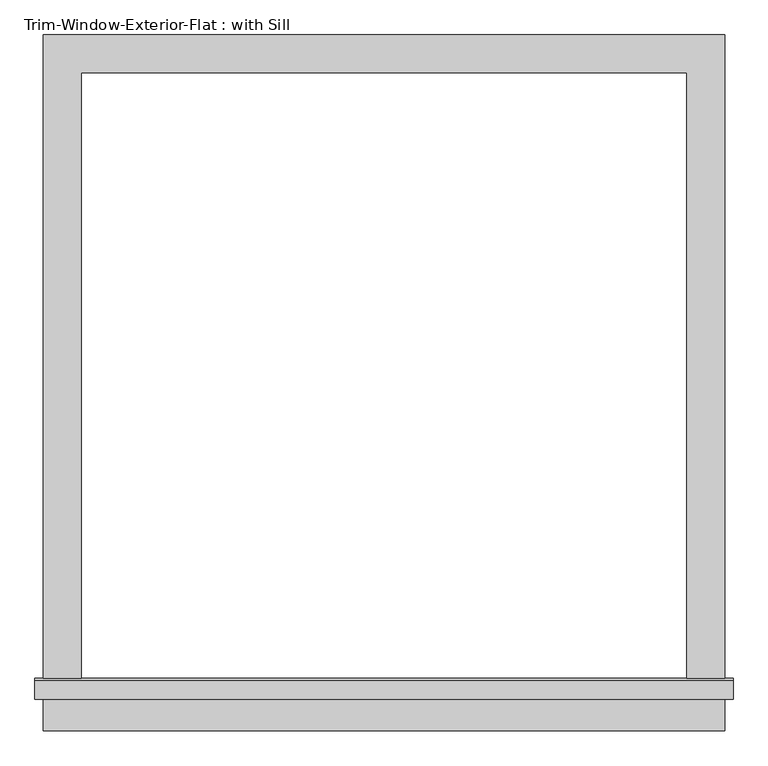
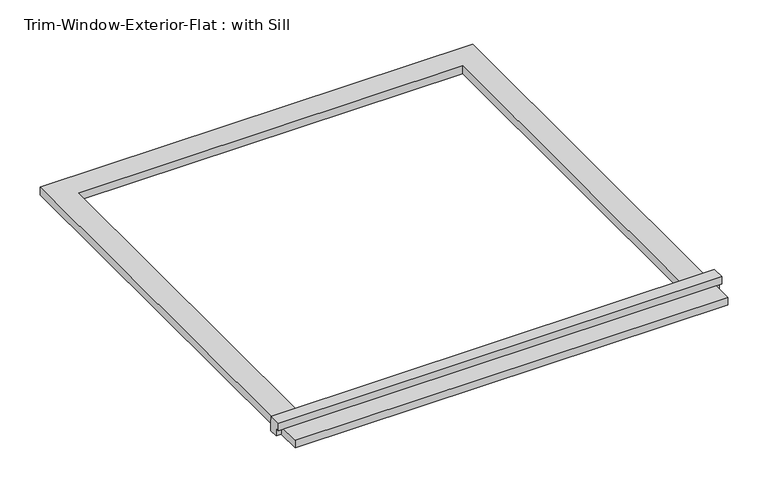
"""IFC4 building model written with IfcOpenShell, lengths in millimetres: proxy geometry, Trim-Window-Exterior-Flat : with Sill."""

from ifc_helpers import new_model, si_unit, frame, origin, origin_with_axes, place, context, project, spatial, polyline, outline, extrude, source, transform, mapped, element, save


def trim_window_exterior_flat_with_sill_84e24481(model_context):
    return source(origin(), model_context, "Body", "SweptSolid", [
        extrude(outline(polyline([(514.35, -936.5823709), (514.35, -993.7323709), (-514.35, -993.7323709), (-514.35, -936.5823709), (514.35, -936.5823709)])), origin_with_axes(), (0.0, 0.0, 1.0), 19.05),
        extrude(outline(polyline([(-946.15, 38.1), (-916.8580645, 38.1), (-914.4, 19.05), (-914.4, 0.0), (-936.5823709, 0.0), (-936.5823709, 19.05), (-946.15, 19.05), (-946.15, 38.1)])), frame((-527.05, 0.0, 0.0), z_axis=(1.0, 0.0, 0.0), x_axis=(0.0, 1.0, 0.0)), (0.0, 0.0, 1.0), 1054.1),
        extrude(outline(polyline([(-514.35, 57.15), (514.35, 57.15), (514.35, -914.4), (457.2, -914.4), (457.2, 0.0), (-457.2, 0.0), (-457.2, -914.4), (-514.35, -914.4), (-514.35, 57.15)])), origin_with_axes(), (0.0, 0.0, 1.0), 19.05),
    ])


if __name__ == "__main__":
    model = new_model("IFC4")
    model_context = context("Model", 3, world=origin())
    ifc_project = project(units=[si_unit("LENGTHUNIT", "METRE", prefix="MILLI")], contexts=[model_context])
    site = spatial("IfcSite", under=ifc_project)
    building = spatial("IfcBuilding", under=site)
    placement = place(None, origin())
    trim_window_exterior_flat_with_sill_shape = trim_window_exterior_flat_with_sill_84e24481(model_context)
    element("IfcBuildingElementProxy", 1, Name="Trim-Window-Exterior-Flat : with Sill", ObjectType="Trim-Window-Exterior-Flat : with Sill", at=placement, inside=building, context=model_context, shape_type="MappedRepresentation", body=[
        mapped(trim_window_exterior_flat_with_sill_shape, transform((0.0, 0.0, 0.0), x_axis=(1.0, 0.0, 0.0), y_axis=(0.0, 1.0, 0.0), z_axis=(0.0, 0.0, 1.0))),
    ])
    save(model, "model.ifc")

# Revit data of these elements
# Type "Trim-Window-Exterior-Flat : with Sill"
#   Trim Width = 0' - 2 1/4"
#   Trim Thickness_Picture Frame = 0' - 1 1/4"
#   Trim Thickness_with Sill = 0' - 0 3/4"
#   Sill Thickness = 0' - 1 1/4"
#   Opening Width [instance default] = 2' - 0"
#   Opening Height [instance default] = 3' - 0"
#   Default Elevation = 4' - 0"
#   Sill = yes
#   Picture Frame = no
#   Trim Material [instance default] = none
# Element 1 (IfcBuildingElementProxy, "Trim-Window-Exterior-Flat : with Sill")
#   Opening Width = 3' - 0"
#   Trim Material = Clad - White
#   Materials on its faces: "Clad - White"
# Materials
#   "Clad - White": class "Wood", colour RGB 242 242 238, transparency 0, Cost = 0
